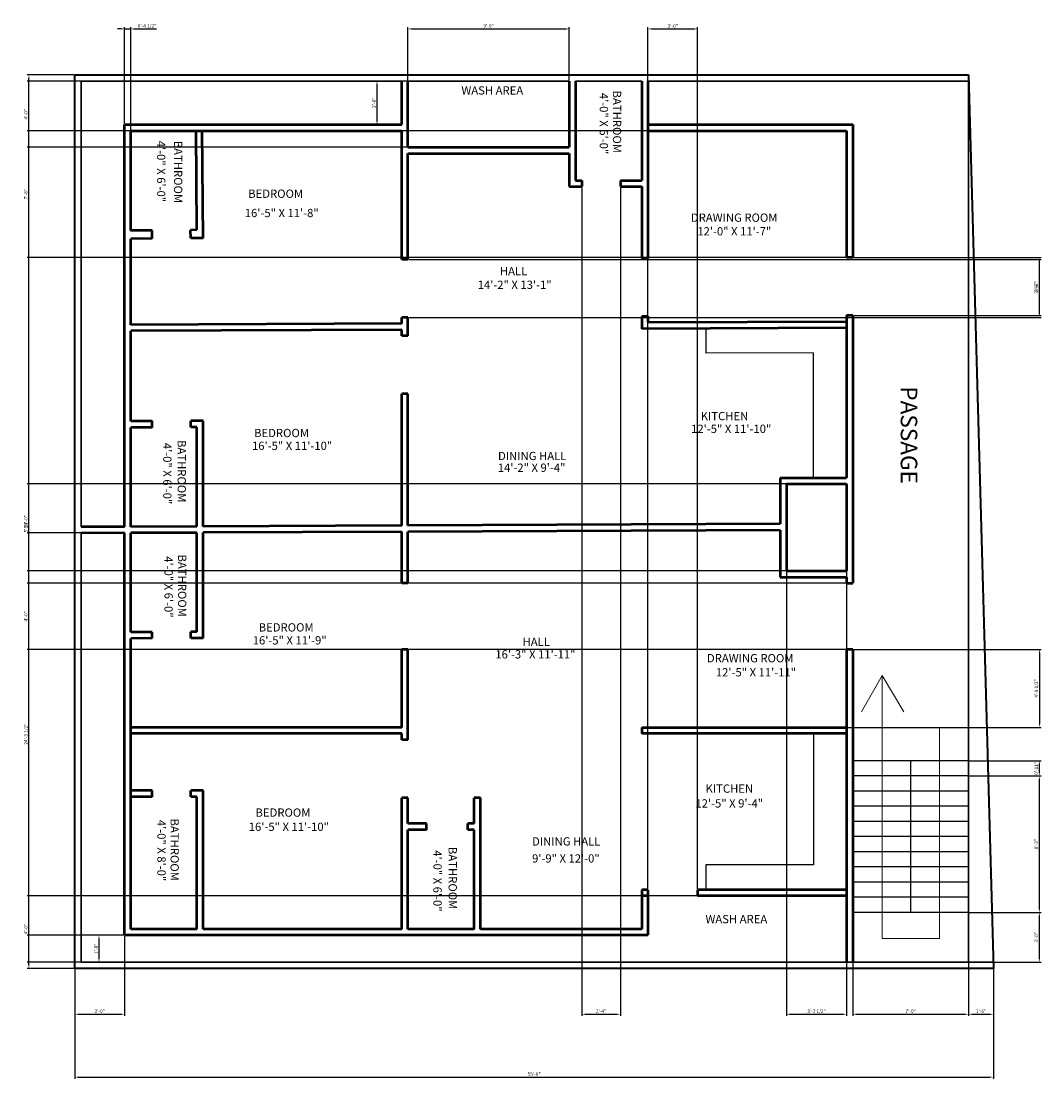
# Model space of a CAD drawing. Units: inches. Extents: x 1269 to 2009, y 1079 to 1846.
import ezdxf

# ---------------------------------------------------------------- set-up
doc = ezdxf.new("R2010")
doc.units = ezdxf.units.IN
for name, color, linetype, lineweight in [('A-ANNO-DIMS', 2, 'Continuous', 18), ('A-ANNO-SYMB', 2, 'Continuous', 18), ('A-ANNO-TEXT', 3, 'Continuous', 18), ('A-AREA-IDEN', 7, 'Continuous', 25), ('A-FLOR-CASE', 9, 'Continuous', 25), ('A-FLOR-STRS', 7, 'Continuous', 25), ('A-WALL', 7, 'Continuous', 50), ('C-PROP', 3, 'Continuous', 35), ('L-SITE-WALL', 8, 'Continuous', 30)]:
    doc.layers.add(name, color=color, linetype=linetype, lineweight=lineweight)
doc.styles.get("Standard").update_dxf_attribs({"font": 'arial.ttf'})
doc.dimstyles.new('ISO-25', dxfattribs={"dimtxt": 2.5, "dimasz": 2.5, "dimexe": 1.25, "dimexo": 0.625, "dimtad": 1, "dimdec": 0, "dimlunit": 4, "dimtxsty": 'Standard', "dimcen": 2.5, "dimadec": 0, "dimazin": 0, "dimtfac": 1, "dimtdec": 0, "dimtmove": 0, "dimatfit": 3, "dimfxl": 1, "dimarcsym": 0})

# ---------------------------------------------------------------- blocks, each defined once
blk = doc.blocks.new('*D1')
at = {"layer": 'A-ANNO-DIMS', "color": 0, "lineweight": -2, "transparency": 16777216}
for p, q in [((1308.03, 1162.83), (1308.03, 1078.8)), ((1974.03, 1162.83), (1974.03, 1078.8)), ((1310.53, 1080.05), (1971.53, 1080.05))]:
    blk.add_line(p, q, dxfattribs=at)
at = {"layer": 'A-ANNO-DIMS', "color": 0, "transparency": 16777216}
for points in [[(1310.53, 1080.47), (1310.53, 1079.64), (1308.03, 1080.05)], [(1971.53, 1080.47), (1971.53, 1079.64), (1974.03, 1080.05)]]:
    blk.add_solid(points, dxfattribs=at)
at = {"layer": 'Defpoints', "color": 0, "transparency": 16777216}
for p in [(1308.03, 1163.45), (1974.03, 1163.45), (1974.03, 1080.05)]:
    blk.add_point(p, dxfattribs=at)
at = {"layer": 'A-ANNO-DIMS', "color": 0, "transparency": 16777216, "insert": (1641.03, 1081.96), "char_height": 2.5, "attachment_point": 5}
blk.add_mtext('55\'-6"', dxfattribs=at)
blk = doc.blocks.new('*D2')
at = {"layer": 'A-ANNO-DIMS', "color": 0, "lineweight": -2, "transparency": 16777216}
for p, q in [((1343.41, 1182.95), (1324.26, 1182.95)), ((1325.51, 1180.45), (1325.51, 1165.95)), ((1343.41, 1163.45), (1324.26, 1163.45))]:
    blk.add_line(p, q, dxfattribs=at)
at = {"layer": 'A-ANNO-DIMS', "color": 0, "transparency": 16777216}
for points in [[(1325.1, 1180.45), (1325.93, 1180.45), (1325.51, 1182.95)], [(1325.1, 1165.95), (1325.93, 1165.95), (1325.51, 1163.45)]]:
    blk.add_solid(points, dxfattribs=at)
at = {"layer": 'Defpoints', "color": 0, "transparency": 16777216}
for p in [(1344.03, 1182.95), (1325.51, 1163.45), (1344.03, 1163.45)]:
    blk.add_point(p, dxfattribs=at)
at = {"layer": 'A-ANNO-DIMS', "color": 0, "transparency": 16777216, "insert": (1323.61, 1173.2), "char_height": 2.5, "attachment_point": 5, "rotation": 90}
blk.add_mtext('1\'-8"', dxfattribs=at)
blk = doc.blocks.new('*D3')
at = {"layer": 'A-ANNO-DIMS', "color": 0, "lineweight": -2, "transparency": 16777216}
for p, q in [((1544.41, 1802.45), (1525.84, 1802.45)), ((1527.09, 1799.95), (1527.09, 1773.45)), ((1544.41, 1770.95), (1525.84, 1770.95))]:
    blk.add_line(p, q, dxfattribs=at)
at = {"layer": 'A-ANNO-DIMS', "color": 0, "transparency": 16777216}
for points in [[(1526.67, 1799.95), (1527.51, 1799.95), (1527.09, 1802.45)], [(1526.67, 1773.45), (1527.51, 1773.45), (1527.09, 1770.95)]]:
    blk.add_solid(points, dxfattribs=at)
at = {"layer": 'Defpoints', "color": 0, "transparency": 16777216}
for p in [(1545.03, 1802.45), (1527.09, 1770.95), (1545.03, 1770.95)]:
    blk.add_point(p, dxfattribs=at)
at = {"layer": 'A-ANNO-DIMS', "color": 0, "transparency": 16777216, "insert": (1525.19, 1786.7), "char_height": 2.5, "attachment_point": 5, "rotation": 90}
blk.add_mtext('2\'-8"', dxfattribs=at)
blk = doc.blocks.new('*D4')
at = {"layer": 'A-ANNO-DIMS', "color": 0, "lineweight": -2, "transparency": 16777216}
for p, q in [((1307.41, 1806.95), (1273.48, 1806.95)), ((1274.73, 1161.45), (1274.73, 1804.45)), ((1307.41, 1158.95), (1273.48, 1158.95))]:
    blk.add_line(p, q, dxfattribs=at)
at = {"layer": 'A-ANNO-DIMS', "color": 0, "transparency": 16777216}
for points in [[(1274.31, 1804.45), (1275.14, 1804.45), (1274.73, 1806.95)], [(1274.31, 1161.45), (1275.14, 1161.45), (1274.73, 1158.95)]]:
    blk.add_solid(points, dxfattribs=at)
at = {"layer": 'Defpoints', "color": 0, "transparency": 16777216}
for p in [(1274.73, 1806.95), (1308.03, 1806.95), (1308.03, 1158.95)]:
    blk.add_point(p, dxfattribs=at)
at = {"layer": 'A-ANNO-DIMS', "color": 0, "transparency": 16777216, "insert": (1272.83, 1482.95), "char_height": 2.5, "attachment_point": 5, "rotation": 90}
blk.add_mtext('54\'-0"', dxfattribs=at)
blk = doc.blocks.new('*D5')
at = {"layer": 'A-ANNO-DIMS', "color": 0, "lineweight": -2, "transparency": 16777216}
for p, q in [((1344.03, 1182.33), (1344.03, 1124.4)), ((1308.03, 1158.33), (1308.03, 1124.4)), ((1310.53, 1125.65), (1341.53, 1125.65))]:
    blk.add_line(p, q, dxfattribs=at)
at = {"layer": 'A-ANNO-DIMS', "color": 0, "transparency": 16777216}
for points in [[(1310.53, 1126.06), (1310.53, 1125.23), (1308.03, 1125.65)], [(1341.53, 1126.06), (1341.53, 1125.23), (1344.03, 1125.65)]]:
    blk.add_solid(points, dxfattribs=at)
at = {"layer": 'Defpoints', "color": 0, "transparency": 16777216}
for p in [(1344.03, 1182.95), (1308.03, 1158.95), (1344.03, 1125.65)]:
    blk.add_point(p, dxfattribs=at)
at = {"layer": 'A-ANNO-DIMS', "color": 0, "transparency": 16777216, "insert": (1326.03, 1127.55), "char_height": 2.5, "attachment_point": 5}
blk.add_mtext('3\'-0"', dxfattribs=at)
blk = doc.blocks.new('*D6')
at = {"layer": 'A-ANNO-DIMS', "color": 0, "lineweight": -2, "transparency": 16777216}
for p, q in [((1872.03, 1162.83), (1872.03, 1124.4)), ((1956.03, 1162.83), (1956.03, 1124.4)), ((1874.53, 1125.65), (1953.53, 1125.65))]:
    blk.add_line(p, q, dxfattribs=at)
at = {"layer": 'A-ANNO-DIMS', "color": 0, "transparency": 16777216}
for points in [[(1874.53, 1126.06), (1874.53, 1125.23), (1872.03, 1125.65)], [(1953.53, 1126.06), (1953.53, 1125.23), (1956.03, 1125.65)]]:
    blk.add_solid(points, dxfattribs=at)
at = {"layer": 'Defpoints', "color": 0, "transparency": 16777216}
for p in [(1872.03, 1163.45), (1956.03, 1163.45), (1956.03, 1125.65)]:
    blk.add_point(p, dxfattribs=at)
at = {"layer": 'A-ANNO-DIMS', "color": 0, "transparency": 16777216, "insert": (1914.03, 1127.55), "char_height": 2.5, "attachment_point": 5}
blk.add_mtext('7\'-0"', dxfattribs=at)
blk = doc.blocks.new('*D7')
at = {"layer": 'A-ANNO-DIMS', "color": 0, "lineweight": -2, "transparency": 16777216}
for p, q in [((1956.03, 1162.83), (1956.03, 1124.4)), ((1974.03, 1162.83), (1974.03, 1124.4)), ((1958.53, 1125.65), (1971.53, 1125.65))]:
    blk.add_line(p, q, dxfattribs=at)
at = {"layer": 'A-ANNO-DIMS', "color": 0, "transparency": 16777216}
for points in [[(1958.53, 1126.06), (1958.53, 1125.23), (1956.03, 1125.65)], [(1971.53, 1126.06), (1971.53, 1125.23), (1974.03, 1125.65)]]:
    blk.add_solid(points, dxfattribs=at)
at = {"layer": 'Defpoints', "color": 0, "transparency": 16777216}
for p in [(1956.03, 1163.45), (1974.03, 1163.45), (1974.03, 1125.65)]:
    blk.add_point(p, dxfattribs=at)
at = {"layer": 'A-ANNO-DIMS', "color": 0, "transparency": 16777216, "insert": (1965.03, 1127.55), "char_height": 2.5, "attachment_point": 5}
blk.add_mtext('1\'-6"', dxfattribs=at)
blk = doc.blocks.new('*D8')
at = {"layer": 'A-ANNO-DIMS', "color": 0, "lineweight": -2, "transparency": 16777216}
for p, q in [((1343.41, 1474.7), (1273.48, 1474.7)), ((1274.73, 1185.45), (1274.73, 1472.2)), ((1343.41, 1182.95), (1273.48, 1182.95))]:
    blk.add_line(p, q, dxfattribs=at)
at = {"layer": 'A-ANNO-DIMS', "color": 0, "transparency": 16777216}
for points in [[(1274.31, 1472.2), (1275.14, 1472.2), (1274.73, 1474.7)], [(1274.31, 1185.45), (1275.14, 1185.45), (1274.73, 1182.95)]]:
    blk.add_solid(points, dxfattribs=at)
at = {"layer": 'Defpoints', "color": 0, "transparency": 16777216}
for p in [(1274.73, 1474.7), (1344.03, 1474.7), (1344.03, 1182.95)]:
    blk.add_point(p, dxfattribs=at)
at = {"layer": 'A-ANNO-DIMS', "color": 0, "transparency": 16777216, "insert": (1272.81, 1328.83), "char_height": 2.5, "attachment_point": 5, "rotation": 90}
blk.add_mtext('24\'-3 1/2"', dxfattribs=at)
blk = doc.blocks.new('*D9')
at = {"layer": 'A-ANNO-DIMS', "color": 0, "lineweight": -2, "transparency": 16777216}
for p, q in [((1956.66, 1298.45), (2008.58, 1298.45)), ((2007.33, 1201.95), (2007.33, 1295.95)), ((1956.66, 1199.45), (2008.58, 1199.45))]:
    blk.add_line(p, q, dxfattribs=at)
at = {"layer": 'A-ANNO-DIMS', "color": 0, "transparency": 16777216}
for points in [[(2006.92, 1295.95), (2007.75, 1295.95), (2007.33, 1298.45)], [(2006.92, 1201.95), (2007.75, 1201.95), (2007.33, 1199.45)]]:
    blk.add_solid(points, dxfattribs=at)
at = {"layer": 'Defpoints', "color": 0, "transparency": 16777216}
for p in [(1956.03, 1298.45), (2007.33, 1298.45), (1956.03, 1199.45)]:
    blk.add_point(p, dxfattribs=at)
at = {"layer": 'A-ANNO-DIMS', "color": 0, "transparency": 16777216, "insert": (2005.43, 1248.95), "char_height": 2.5, "attachment_point": 5, "rotation": 90}
blk.add_mtext('8\'-3"', dxfattribs=at)
blk = doc.blocks.new('*D10')
at = {"layer": 'A-ANNO-DIMS', "color": 0, "lineweight": -2, "transparency": 16777216}
for p, q in [((1956.66, 1199.45), (2008.58, 1199.45)), ((2007.33, 1165.95), (2007.33, 1196.95)), ((1956.66, 1163.45), (2008.58, 1163.45))]:
    blk.add_line(p, q, dxfattribs=at)
at = {"layer": 'A-ANNO-DIMS', "color": 0, "transparency": 16777216}
for points in [[(2006.92, 1196.95), (2007.75, 1196.95), (2007.33, 1199.45)], [(2006.92, 1165.95), (2007.75, 1165.95), (2007.33, 1163.45)]]:
    blk.add_solid(points, dxfattribs=at)
at = {"layer": 'Defpoints', "color": 0, "transparency": 16777216}
for p in [(1956.03, 1199.45), (2007.33, 1199.45), (1956.03, 1163.45)]:
    blk.add_point(p, dxfattribs=at)
at = {"layer": 'A-ANNO-DIMS', "color": 0, "transparency": 16777216, "insert": (2005.43, 1181.45), "char_height": 2.5, "attachment_point": 5, "rotation": 90}
blk.add_mtext('3\'-0"', dxfattribs=at)
blk = doc.blocks.new('*D11')
at = {"layer": 'A-ANNO-DIMS', "color": 0, "lineweight": -2, "transparency": 16777216}
for p, q in [((1872.66, 1674.45), (2008.58, 1674.45)), ((2007.33, 1634.95), (2007.33, 1671.95)), ((1872.66, 1632.45), (2008.58, 1632.45))]:
    blk.add_line(p, q, dxfattribs=at)
at = {"layer": 'A-ANNO-DIMS', "color": 0, "transparency": 16777216}
for points in [[(2006.92, 1671.95), (2007.75, 1671.95), (2007.33, 1674.45)], [(2006.92, 1634.95), (2007.75, 1634.95), (2007.33, 1632.45)]]:
    blk.add_solid(points, dxfattribs=at)
at = {"layer": 'Defpoints', "color": 0, "transparency": 16777216}
for p in [(1872.03, 1674.45), (2007.33, 1674.45), (1872.03, 1632.45)]:
    blk.add_point(p, dxfattribs=at)
at = {"layer": 'A-ANNO-DIMS', "color": 0, "transparency": 16777216, "insert": (2005.43, 1653.45), "char_height": 2.5, "attachment_point": 5, "rotation": 90}
blk.add_mtext('3\'-6"', dxfattribs=at)
blk = doc.blocks.new('*D12')
at = {"layer": 'A-ANNO-DIMS', "color": 0, "lineweight": -2, "transparency": 16777216}
for p, q in [((1866.91, 1766.45), (1273.48, 1766.45)), ((1274.73, 1676.93), (1274.73, 1763.95)), ((1866.91, 1674.43), (1273.48, 1674.43))]:
    blk.add_line(p, q, dxfattribs=at)
at = {"layer": 'A-ANNO-DIMS', "color": 0, "transparency": 16777216}
for points in [[(1274.31, 1763.95), (1275.14, 1763.95), (1274.73, 1766.45)], [(1274.31, 1676.93), (1275.14, 1676.93), (1274.73, 1674.43)]]:
    blk.add_solid(points, dxfattribs=at)
at = {"layer": 'Defpoints', "color": 0, "transparency": 16777216}
for p in [(1274.73, 1766.45), (1867.53, 1766.45), (1867.53, 1674.43)]:
    blk.add_point(p, dxfattribs=at)
at = {"layer": 'A-ANNO-DIMS', "color": 0, "transparency": 16777216, "insert": (1272.83, 1720.44), "char_height": 2.5, "attachment_point": 5, "rotation": 90}
blk.add_mtext('7\'-8"', dxfattribs=at)
blk = doc.blocks.new('*D13')
at = {"layer": 'A-ANNO-DIMS', "color": 0, "lineweight": -2, "transparency": 16777216}
for p, q in [((1866.91, 1438.27), (1273.48, 1438.27)), ((1274.73, 1392.77), (1274.73, 1435.77)), ((1866.91, 1390.27), (1273.48, 1390.27))]:
    blk.add_line(p, q, dxfattribs=at)
at = {"layer": 'A-ANNO-DIMS', "color": 0, "transparency": 16777216}
for points in [[(1274.31, 1435.77), (1275.14, 1435.77), (1274.73, 1438.27)], [(1274.31, 1392.77), (1275.14, 1392.77), (1274.73, 1390.27)]]:
    blk.add_solid(points, dxfattribs=at)
at = {"layer": 'Defpoints', "color": 0, "transparency": 16777216}
for p in [(1274.73, 1438.27), (1867.53, 1438.27), (1867.53, 1390.27)]:
    blk.add_point(p, dxfattribs=at)
at = {"layer": 'A-ANNO-DIMS', "color": 0, "transparency": 16777216, "insert": (1272.83, 1414.27), "char_height": 2.5, "attachment_point": 5, "rotation": 90}
blk.add_mtext('4\'-0"', dxfattribs=at)
blk = doc.blocks.new('*D14')
at = {"layer": 'A-ANNO-DIMS', "color": 0, "lineweight": -2, "transparency": 16777216}
for p, q in [((1868.16, 1390.27), (2008.58, 1390.27)), ((2007.33, 1387.77), (2007.33, 1336.2)), ((1868.16, 1333.7), (2008.58, 1333.7))]:
    blk.add_line(p, q, dxfattribs=at)
at = {"layer": 'A-ANNO-DIMS', "color": 0, "transparency": 16777216}
for points in [[(2006.92, 1387.77), (2007.75, 1387.77), (2007.33, 1390.27)], [(2006.92, 1336.2), (2007.75, 1336.2), (2007.33, 1333.7)]]:
    blk.add_solid(points, dxfattribs=at)
at = {"layer": 'Defpoints', "color": 0, "transparency": 16777216}
for p in [(1867.53, 1390.27), (1867.53, 1333.7), (2007.33, 1333.7)]:
    blk.add_point(p, dxfattribs=at)
at = {"layer": 'A-ANNO-DIMS', "color": 0, "transparency": 16777216, "insert": (2005.42, 1361.99), "char_height": 2.5, "attachment_point": 5, "rotation": 90}
blk.add_mtext('4\'-8 1/2"', dxfattribs=at)
blk = doc.blocks.new('*D15')
at = {"layer": 'A-ANNO-DIMS', "color": 0, "lineweight": -2, "transparency": 16777216}
for p, q in [((1675.53, 1725.33), (1675.53, 1124.4)), ((1703.53, 1725.33), (1703.53, 1124.4)), ((1678.03, 1125.65), (1701.03, 1125.65))]:
    blk.add_line(p, q, dxfattribs=at)
at = {"layer": 'A-ANNO-DIMS', "color": 0, "transparency": 16777216}
for points in [[(1678.03, 1126.06), (1678.03, 1125.23), (1675.53, 1125.65)], [(1701.03, 1126.06), (1701.03, 1125.23), (1703.53, 1125.65)]]:
    blk.add_solid(points, dxfattribs=at)
at = {"layer": 'Defpoints', "color": 0, "transparency": 16777216}
for p in [(1675.53, 1725.95), (1703.53, 1725.95), (1703.53, 1125.65)]:
    blk.add_point(p, dxfattribs=at)
at = {"layer": 'A-ANNO-DIMS', "color": 0, "transparency": 16777216, "insert": (1689.53, 1127.53), "char_height": 2.5, "attachment_point": 5}
blk.add_mtext('2\'-4"', dxfattribs=at)
blk = doc.blocks.new('*D16')
at = {"layer": 'A-ANNO-DIMS', "color": 0, "lineweight": -2, "transparency": 16777216}
for p, q in [((1549.53, 1803.08), (1549.53, 1841.5)), ((1666.53, 1803.08), (1666.53, 1841.5)), ((1552.03, 1840.25), (1664.03, 1840.25))]:
    blk.add_line(p, q, dxfattribs=at)
at = {"layer": 'A-ANNO-DIMS', "color": 0, "transparency": 16777216}
for points in [[(1552.03, 1840.67), (1552.03, 1839.84), (1549.53, 1840.25)], [(1664.03, 1840.67), (1664.03, 1839.84), (1666.53, 1840.25)]]:
    blk.add_solid(points, dxfattribs=at)
at = {"layer": 'Defpoints', "color": 0, "transparency": 16777216}
for p in [(1666.53, 1840.25), (1549.53, 1802.45), (1666.53, 1802.45)]:
    blk.add_point(p, dxfattribs=at)
at = {"layer": 'A-ANNO-DIMS', "color": 0, "transparency": 16777216, "insert": (1608.03, 1842.16), "char_height": 2.5, "attachment_point": 5}
blk.add_mtext('9\'-9"', dxfattribs=at)
blk = doc.blocks.new('*D17')
at = {"layer": 'A-ANNO-DIMS', "color": 0, "lineweight": -2, "transparency": 16777216}
for p, q in [((1665.91, 1802.45), (1273.48, 1802.45)), ((1274.73, 1756.95), (1274.73, 1799.95)), ((1665.91, 1754.45), (1273.48, 1754.45))]:
    blk.add_line(p, q, dxfattribs=at)
at = {"layer": 'A-ANNO-DIMS', "color": 0, "transparency": 16777216}
for points in [[(1274.31, 1799.95), (1275.14, 1799.95), (1274.73, 1802.45)], [(1274.31, 1756.95), (1275.14, 1756.95), (1274.73, 1754.45)]]:
    blk.add_solid(points, dxfattribs=at)
at = {"layer": 'Defpoints', "color": 0, "transparency": 16777216}
for p in [(1274.73, 1802.45), (1666.53, 1802.45), (1666.53, 1754.45)]:
    blk.add_point(p, dxfattribs=at)
at = {"layer": 'A-ANNO-DIMS', "color": 0, "transparency": 16777216, "insert": (1272.83, 1778.45), "char_height": 2.5, "attachment_point": 5, "rotation": 90}
blk.add_mtext('4\'-0"', dxfattribs=at)
blk = doc.blocks.new('*D18')
at = {"layer": 'A-ANNO-DIMS', "color": 0, "lineweight": -2, "transparency": 16777216}
for p, q in [((1723.53, 1216.58), (1723.53, 1841.5)), ((1759.53, 1216.58), (1759.53, 1841.5)), ((1726.03, 1840.25), (1757.03, 1840.25))]:
    blk.add_line(p, q, dxfattribs=at)
at = {"layer": 'A-ANNO-DIMS', "color": 0, "transparency": 16777216}
for points in [[(1726.03, 1840.67), (1726.03, 1839.84), (1723.53, 1840.25)], [(1757.03, 1840.67), (1757.03, 1839.84), (1759.53, 1840.25)]]:
    blk.add_solid(points, dxfattribs=at)
at = {"layer": 'Defpoints', "color": 0, "transparency": 16777216}
for p in [(1759.53, 1840.25), (1723.53, 1215.95), (1759.53, 1215.95)]:
    blk.add_point(p, dxfattribs=at)
at = {"layer": 'A-ANNO-DIMS', "color": 0, "transparency": 16777216, "insert": (1741.53, 1842.16), "char_height": 2.5, "attachment_point": 5}
blk.add_mtext('3\'-0"', dxfattribs=at)
blk = doc.blocks.new('*D19')
at = {"layer": 'A-ANNO-DIMS', "color": 0, "lineweight": -2, "transparency": 16777216}
for p, q in [((1956.66, 1309.45), (2008.58, 1309.45)), ((2007.33, 1300.95), (2007.33, 1306.95)), ((1956.66, 1298.45), (2008.58, 1298.45))]:
    blk.add_line(p, q, dxfattribs=at)
at = {"layer": 'A-ANNO-DIMS', "color": 0, "transparency": 16777216}
for points in [[(2006.92, 1306.95), (2007.75, 1306.95), (2007.33, 1309.45)], [(2006.92, 1300.95), (2007.75, 1300.95), (2007.33, 1298.45)]]:
    blk.add_solid(points, dxfattribs=at)
at = {"layer": 'Defpoints', "color": 0, "transparency": 16777216}
for p in [(1956.03, 1309.45), (2007.33, 1309.45), (1956.03, 1298.45)]:
    blk.add_point(p, dxfattribs=at)
at = {"layer": 'A-ANNO-DIMS', "color": 0, "transparency": 16777216, "insert": (2005.43, 1303.95), "char_height": 2.5, "attachment_point": 5, "rotation": 90}
blk.add_mtext('0\'-11"', dxfattribs=at)
blk = doc.blocks.new('*D20')
at = {"layer": 'A-ANNO-DIMS', "color": 0, "lineweight": -2, "transparency": 16777216}
for p, q in [((1344.03, 1771.58), (1344.03, 1841.5)), ((1348.53, 1767.08), (1348.53, 1841.5)), ((1341.53, 1840.25), (1339.03, 1840.25)), ((1344.03, 1840.25), (1348.53, 1840.25)), ((1351.03, 1840.25), (1367.25, 1840.25))]:
    blk.add_line(p, q, dxfattribs=at)
at = {"layer": 'A-ANNO-DIMS', "color": 0, "transparency": 16777216}
for points in [[(1341.53, 1840.67), (1341.53, 1839.84), (1344.03, 1840.25)], [(1351.03, 1840.67), (1351.03, 1839.84), (1348.53, 1840.25)]]:
    blk.add_solid(points, dxfattribs=at)
at = {"layer": 'Defpoints', "color": 0, "transparency": 16777216}
for p in [(1348.53, 1840.25), (1344.03, 1770.95), (1348.53, 1766.45)]:
    blk.add_point(p, dxfattribs=at)
at = {"layer": 'A-ANNO-DIMS', "color": 0, "transparency": 16777216, "insert": (1360.39, 1842.17), "char_height": 2.5, "attachment_point": 5}
blk.add_mtext('0\'-4 1/2"', dxfattribs=at)
blk = doc.blocks.new('*D21')
at = {"layer": 'A-ANNO-DIMS', "color": 0, "lineweight": -2, "transparency": 16777216}
for p, q in [((1824.03, 1509.65), (1824.03, 1124.4)), ((1867.53, 1509.65), (1867.53, 1124.4)), ((1826.53, 1125.65), (1865.03, 1125.65))]:
    blk.add_line(p, q, dxfattribs=at)
at = {"layer": 'A-ANNO-DIMS', "color": 0, "transparency": 16777216}
for points in [[(1826.53, 1126.06), (1826.53, 1125.23), (1824.03, 1125.65)], [(1865.03, 1126.06), (1865.03, 1125.23), (1867.53, 1125.65)]]:
    blk.add_solid(points, dxfattribs=at)
at = {"layer": 'Defpoints', "color": 0, "transparency": 16777216}
for p in [(1824.03, 1510.27), (1867.53, 1510.27), (1867.53, 1125.65)]:
    blk.add_point(p, dxfattribs=at)
at = {"layer": 'A-ANNO-DIMS', "color": 0, "transparency": 16777216, "insert": (1845.78, 1127.57), "char_height": 2.5, "attachment_point": 5}
blk.add_mtext('3\'-7 1/2"', dxfattribs=at)
blk = doc.blocks.new('*D22')
at = {"layer": 'A-ANNO-DIMS', "color": 0, "lineweight": -2, "transparency": 16777216}
for p, q in [((1866.91, 1510.27), (1273.48, 1510.27)), ((1274.73, 1449.77), (1274.73, 1507.77)), ((1866.91, 1447.27), (1273.48, 1447.27))]:
    blk.add_line(p, q, dxfattribs=at)
at = {"layer": 'A-ANNO-DIMS', "color": 0, "transparency": 16777216}
for points in [[(1274.31, 1507.77), (1275.14, 1507.77), (1274.73, 1510.27)], [(1274.31, 1449.77), (1275.14, 1449.77), (1274.73, 1447.27)]]:
    blk.add_solid(points, dxfattribs=at)
at = {"layer": 'Defpoints', "color": 0, "transparency": 16777216}
for p in [(1274.73, 1510.27), (1867.53, 1510.27), (1867.53, 1447.27)]:
    blk.add_point(p, dxfattribs=at)
at = {"layer": 'A-ANNO-DIMS', "color": 0, "transparency": 16777216, "insert": (1272.83, 1478.77), "char_height": 2.5, "attachment_point": 5, "rotation": 90}
blk.add_mtext('5\'-3"', dxfattribs=at)
blk = doc.blocks.new('*D23')
at = {"layer": 'A-ANNO-DIMS', "color": 0, "lineweight": -2, "transparency": 16777216}
for p, q in [((1866.91, 1211.45), (1273.48, 1211.45)), ((1274.73, 1165.95), (1274.73, 1208.95)), ((1866.91, 1163.45), (1273.48, 1163.45))]:
    blk.add_line(p, q, dxfattribs=at)
at = {"layer": 'A-ANNO-DIMS', "color": 0, "transparency": 16777216}
for points in [[(1274.31, 1208.95), (1275.14, 1208.95), (1274.73, 1211.45)], [(1274.31, 1165.95), (1275.14, 1165.95), (1274.73, 1163.45)]]:
    blk.add_solid(points, dxfattribs=at)
at = {"layer": 'Defpoints', "color": 0, "transparency": 16777216}
for p in [(1274.73, 1211.45), (1867.53, 1211.45), (1867.53, 1163.45)]:
    blk.add_point(p, dxfattribs=at)
at = {"layer": 'A-ANNO-DIMS', "color": 0, "transparency": 16777216, "insert": (1272.83, 1187.45), "char_height": 2.5, "attachment_point": 5, "rotation": 90}
blk.add_mtext('4\'-0"', dxfattribs=at)
blk = doc.blocks.new('*D24')
at = {"layer": 'A-ANNO-DIMS', "color": 0, "lineweight": -2, "transparency": 16777216}
for p, q in [((1550.16, 1673.08), (2008.58, 1673.08)), ((2007.33, 1633.58), (2007.33, 1670.58)), ((1550.16, 1631.08), (2008.58, 1631.08))]:
    blk.add_line(p, q, dxfattribs=at)
at = {"layer": 'A-ANNO-DIMS', "color": 0, "transparency": 16777216}
for points in [[(2006.92, 1670.58), (2007.75, 1670.58), (2007.33, 1673.08)], [(2006.92, 1633.58), (2007.75, 1633.58), (2007.33, 1631.08)]]:
    blk.add_solid(points, dxfattribs=at)
at = {"layer": 'Defpoints', "color": 0, "transparency": 16777216}
for p in [(1549.53, 1673.08), (2007.33, 1673.08), (1549.53, 1631.08)]:
    blk.add_point(p, dxfattribs=at)
at = {"layer": 'A-ANNO-DIMS', "color": 0, "transparency": 16777216, "insert": (2005.43, 1652.08), "char_height": 2.5, "attachment_point": 5, "rotation": 90}
blk.add_mtext('3\'-6"', dxfattribs=at)

msp = doc.modelspace()

# ---------------------------------------------------------------- linework, layer by layer
at = {"layer": 'A-ANNO-SYMB'}
for p, q in [((1893.29, 1371.22), (1878.37, 1344.95)), ((1893.29, 1180.65), (1893.29, 1371.22)), ((1893.29, 1371.22), (1909.09, 1345.09)), ((1934.88, 1333.66), (1934.88, 1180.65)), ((1934.88, 1180.65), (1893.29, 1180.65))]:
    msp.add_line(p, q, dxfattribs=at)
at = {"layer": 'A-FLOR-CASE'}
for p, q in [((1765.4, 1623), (1765.4, 1605)), ((1843.4, 1605.33), (1765.4, 1605)), ((1843.4, 1605.33), (1843.4, 1514.77)), ((1843.53, 1329.2), (1843.53, 1233.95)), ((1843.53, 1233.95), (1765.53, 1233.95)), ((1765.53, 1233.95), (1765.53, 1215.95))]:
    msp.add_line(p, q, dxfattribs=at)
at = {"layer": 'A-FLOR-STRS'}
for p, q in [((1956.03, 1309.45), (1872.03, 1309.45)), ((1914.03, 1309.45), (1914.03, 1199.45)), ((1956.03, 1298.45), (1872.03, 1298.45)), ((1956.03, 1287.45), (1872.03, 1287.45)), ((1956.03, 1276.45), (1872.03, 1276.45)), ((1956.03, 1265.45), (1872.03, 1265.45)), ((1956.03, 1254.45), (1872.03, 1254.45)), ((1956.03, 1243.45), (1872.03, 1243.45)), ((1956.03, 1232.45), (1872.03, 1232.45)), ((1956.03, 1221.45), (1872.03, 1221.45)), ((1956.03, 1210.45), (1872.03, 1210.45)), ((1956.03, 1199.45), (1872.03, 1199.45))]:
    msp.add_line(p, q, dxfattribs=at)
at = {"layer": 'A-WALL'}
for p, q in [((1545.03, 1770.95), (1545.03, 1802.45)), ((1549.53, 1754.45), (1549.53, 1802.45)), ((1666.53, 1802.45), (1666.53, 1754.45)), ((1671.03, 1802.45), (1671.03, 1730.45)), ((1719.03, 1802.45), (1719.03, 1730.45)), ((1723.53, 1802.45), (1723.53, 1673.82)), ((1344.03, 1479.2), (1344.03, 1770.95)), ((1344.03, 1770.95), (1545.03, 1770.95)), ((1348.53, 1694.04), (1348.53, 1766.45)), ((1348.53, 1766.45), (1545.03, 1766.45)), ((1396.48, 1694.45), (1395.86, 1766.45)), ((1401.03, 1688.49), (1400.36, 1766.49)), ((1545.03, 1673.06), (1545.03, 1766.45)), ((1723.53, 1770.95), (1872.03, 1770.95)), ((1723.53, 1766.45), (1867.53, 1766.45)), ((1867.53, 1766.45), (1867.53, 1674.43)), ((1872.03, 1770.95), (1872.03, 1674.45)), ((1549.53, 1754.45), (1666.53, 1754.45)), ((1549.53, 1673.08), (1549.53, 1749.95)), ((1549.53, 1749.95), (1666.53, 1749.95)), ((1666.53, 1749.95), (1666.53, 1725.95)), ((1671.03, 1730.45), (1675.53, 1730.45)), ((1675.53, 1730.45), (1675.53, 1725.95)), ((1703.53, 1730.45), (1719.03, 1730.45)), ((1703.53, 1730.45), (1703.53, 1725.95)), ((1666.53, 1725.95), (1675.53, 1725.95)), ((1703.53, 1725.95), (1719.03, 1725.95)), ((1719.03, 1725.95), (1719.03, 1673.8)), ((1363.98, 1694.18), (1348.48, 1694.04)), ((1364.03, 1688.18), (1348.53, 1688.04)), ((1348.53, 1625.72), (1348.53, 1688.04)), ((1364.03, 1688.18), (1363.98, 1694.18)), ((1396.48, 1694.45), (1391.98, 1694.41)), ((1392.03, 1688.42), (1391.98, 1694.41)), ((1401.03, 1688.49), (1392.03, 1688.42)), ((1549.53, 1673.08), (1545.03, 1673.06)), ((1723.53, 1673.82), (1719.03, 1673.8)), ((1872.03, 1674.45), (1867.53, 1674.43)), ((1545.03, 1626.56), (1348.53, 1625.72)), ((1549.53, 1631.08), (1545.03, 1631.06)), ((1545.03, 1626.56), (1545.03, 1631.06)), ((1549.53, 1617.58), (1549.53, 1631.08)), ((1723.53, 1631.82), (1719.03, 1631.8)), ((1719.03, 1631.8), (1719.03, 1622.8)), ((1723.53, 1631.82), (1723.53, 1627.32)), ((1867.53, 1627.93), (1723.53, 1627.32)), ((1872.03, 1632.45), (1867.53, 1632.43)), ((1867.53, 1632.43), (1867.53, 1514.77)), ((1872.03, 1632.45), (1872.03, 1438.27)), ((1545.03, 1622.06), (1348.53, 1621.22)), ((1348.53, 1555.72), (1348.53, 1621.22)), ((1545.03, 1617.56), (1545.03, 1622.06)), ((1867.53, 1623.43), (1719.03, 1622.8)), ((1549.53, 1617.58), (1545.03, 1617.56)), ((1549.53, 1575.58), (1545.03, 1575.56)), ((1545.03, 1480.06), (1545.03, 1575.56)), ((1549.53, 1480.08), (1549.53, 1575.58)), ((1364.03, 1555.79), (1348.53, 1555.72)), ((1364.03, 1551.29), (1348.53, 1551.22)), ((1348.53, 1479.22), (1348.53, 1551.22)), ((1364.03, 1551.29), (1364.03, 1555.93)), ((1401.13, 1555.94), (1392.03, 1555.91)), ((1392.03, 1551.41), (1392.03, 1555.93)), ((1396.53, 1551.43), (1392.03, 1551.41)), ((1396.53, 1479.42), (1396.53, 1551.43)), ((1401.03, 1479.44), (1401.03, 1555.94)), ((1401.13, 1551.44), (1401.03, 1551.44)), ((1819.53, 1514.77), (1819.53, 1481.23)), ((1819.53, 1514.77), (1867.53, 1514.77)), ((1824.03, 1510.27), (1824.03, 1447.27)), ((1824.03, 1510.27), (1867.53, 1510.27)), ((1867.53, 1510.27), (1867.53, 1447.27)), ((1819.53, 1481.23), (1549.53, 1480.08)), ((1344.03, 1479.2), (1312.53, 1479.07)), ((1344.03, 1474.7), (1312.53, 1474.57)), ((1344.03, 1479.2), (1344.02, 1479.2)), ((1344.03, 1182.95), (1344.03, 1474.7)), ((1396.53, 1479.42), (1348.53, 1479.22)), ((1396.53, 1474.92), (1348.53, 1474.72)), ((1348.53, 1402.72), (1348.53, 1474.72)), ((1396.53, 1402.92), (1396.53, 1474.92)), ((1545.03, 1480.06), (1401.03, 1479.44)), ((1545.03, 1475.56), (1401.03, 1474.94)), ((1401.03, 1398.44), (1401.03, 1474.94)), ((1545.03, 1438.27), (1545.03, 1475.56)), ((1819.53, 1476.73), (1549.53, 1475.58)), ((1549.53, 1438.27), (1549.53, 1475.58)), ((1819.53, 1476.73), (1819.53, 1442.77)), ((1872.04, 1476.95), (1872.03, 1476.95)), ((1867.63, 1452.93), (1867.53, 1452.93)), ((1819.53, 1442.77), (1867.53, 1442.77)), ((1824.03, 1447.27), (1867.53, 1447.27)), ((1867.53, 1442.77), (1867.53, 1438.27)), ((1549.53, 1438.27), (1545.03, 1438.27)), ((1867.53, 1438.27), (1872.03, 1438.27)), ((1364.03, 1402.79), (1348.53, 1402.72)), ((1364.03, 1398.29), (1348.53, 1398.22)), ((1348.53, 1187.45), (1348.53, 1398.22)), ((1364.03, 1398.29), (1364.03, 1402.79)), ((1396.53, 1402.92), (1392.03, 1402.9)), ((1392.03, 1398.4), (1392.03, 1402.9)), ((1401.03, 1398.44), (1392.03, 1398.4)), ((1545.03, 1333.7), (1545.03, 1390.27)), ((1549.53, 1390.27), (1545.03, 1390.27)), ((1549.53, 1324.7), (1549.53, 1390.27)), ((1867.53, 1390.27), (1867.53, 1163.45)), ((1872.03, 1390.27), (1867.53, 1390.27)), ((1872.03, 1390.27), (1872.03, 1163.45)), ((1545.03, 1333.7), (1348.53, 1333.7)), ((1545.03, 1329.2), (1348.53, 1329.2)), ((1545.03, 1324.7), (1545.03, 1329.2)), ((1719.03, 1333.7), (1719.03, 1329.2)), ((1719.03, 1333.7), (1867.53, 1333.7)), ((1867.53, 1329.2), (1719.03, 1329.2)), ((1767.04, 1333.7), (1771.54, 1333.7)), ((1549.53, 1324.7), (1545.03, 1324.7)), ((1364.03, 1287.95), (1348.53, 1287.95)), ((1364.03, 1283.45), (1348.53, 1283.45)), ((1364.03, 1283.45), (1364.03, 1287.95)), ((1401.03, 1287.95), (1392.03, 1287.95)), ((1392.03, 1283.45), (1392.03, 1287.95)), ((1396.53, 1283.45), (1392.03, 1283.45)), ((1396.53, 1187.45), (1396.53, 1283.45)), ((1401.03, 1187.45), (1401.03, 1287.95)), ((1549.53, 1282.7), (1545.03, 1282.7)), ((1545.03, 1187.45), (1545.03, 1282.7)), ((1549.53, 1263.95), (1549.53, 1282.7)), ((1602.03, 1282.7), (1597.53, 1282.7)), ((1597.53, 1263.95), (1597.53, 1282.7)), ((1602.03, 1187.45), (1602.03, 1282.7)), ((1563.03, 1263.95), (1549.53, 1263.95)), ((1563.03, 1259.45), (1549.53, 1259.45)), ((1549.53, 1187.45), (1549.53, 1259.45)), ((1563.03, 1259.45), (1563.03, 1263.95)), ((1597.53, 1263.95), (1593.03, 1263.95)), ((1593.03, 1259.45), (1593.03, 1263.95)), ((1597.53, 1259.45), (1593.03, 1259.45)), ((1597.53, 1187.45), (1597.53, 1259.45)), ((1723.53, 1215.95), (1719.03, 1215.95)), ((1719.03, 1215.95), (1719.03, 1187.45)), ((1723.53, 1215.95), (1723.53, 1182.95)), ((1867.53, 1215.95), (1759.53, 1215.95)), ((1759.53, 1215.95), (1759.53, 1211.45)), ((1723.53, 1211.45), (1719.03, 1211.45)), ((1867.53, 1211.45), (1759.53, 1211.45)), ((1723.53, 1182.95), (1344.03, 1182.95)), ((1396.53, 1187.45), (1348.53, 1187.45)), ((1545.03, 1187.45), (1401.03, 1187.45)), ((1597.53, 1187.45), (1549.53, 1187.45)), ((1719.03, 1187.45), (1602.03, 1187.45))]:
    msp.add_line(p, q, dxfattribs=at)
at = {"layer": 'C-PROP'}
for p, q in [((1308.03, 1158.95), (1308.03, 1806.95)), ((1308.03, 1806.95), (1956.03, 1806.95)), ((1956.03, 1806.95), (1974.03, 1158.95)), ((1974.03, 1158.95), (1308.03, 1158.95))]:
    msp.add_line(p, q, dxfattribs=at)
at = {"layer": 'L-SITE-WALL'}
for p, q in [((1956.03, 1806.95), (1956.03, 1163.45)), ((1312.53, 1479.07), (1312.53, 1802.45)), ((1312.53, 1802.45), (1545.03, 1802.45)), ((1549.53, 1802.45), (1666.53, 1802.45)), ((1671.03, 1802.45), (1719.03, 1802.45)), ((1723.53, 1802.45), (1956.03, 1802.45)), ((1312.53, 1163.45), (1312.53, 1474.57)), ((1974.03, 1163.45), (1312.53, 1163.45))]:
    msp.add_line(p, q, dxfattribs=at)

# ---------------------------------------------------------------- texts
at = {"layer": 'A-ANNO-TEXT', "char_height": 6, "attachment_point": 1, "rotation": 270}
for s, width, insert in [('4\'-0" X 6\'-0"', 45.2228, (1694.59, 1793.9)), ('4\'-0" X 6\'-0"', 45.2228, (1373.57, 1759.17)), ('4\'-0" X 6\'-0"', 45.2228, (1378.07, 1540.05)), ('4\'-0" X 6\'-0"', 45.2228, (1378.99, 1457.83)), ('4\'-0" X 8\'-0"', 47.7154, (1373.86, 1266.64)), ('4\'-0" X 6\'-0"', 45.2228, (1573.99, 1244.61))]:
    msp.add_mtext_dynamic_manual_height_columns(s, width=width, gutter_width=12.5, heights=[0], dxfattribs=dict(at, insert=insert))
at = {"layer": 'A-ANNO-TEXT', "char_height": 6, "attachment_point": 1}
for s, width, insert in [('16\'-5" X 11\'-8"', 58.2006, (1431.23, 1709.75)), ('12\'-0" X 11\'-7"', 53.9923, (1759.35, 1696.5)), ('14\'-2" X 13\'-1"', 53.9923, (1600.09, 1657.68)), ('12\'-5" X 11\'-10"', 61.4849, (1754.85, 1553.22)), ('16\'-5" X 11\'-10"', 66.6765, (1436.46, 1540.92)), ('14\'-2" X 9\'-4"', 53.9923, (1614.66, 1525.04)), ('16\'-5" X 11\'-9"', 53.9923, (1436.99, 1399.83)), ('16\'-3" X 11\'-11"', 67.0938, (1612.88, 1389.69)), ('12\'-5" X 11\'-11"', 67.0938, (1772.79, 1376.67)), ('12\'-5" X 9\'-4"', 53.9923, (1757.98, 1281.58)), ('16\'-5" X 11\'-10"', 66.5223, (1434.11, 1264.61)), ('9\'-9" X 12\'-0"', 53.9923, (1639.52, 1241.66))]:
    msp.add_mtext_dynamic_manual_height_columns(s, width=width, gutter_width=12.5, heights=[0], dxfattribs=dict(at, insert=insert))
at = {"layer": 'A-AREA-IDEN', "char_height": 6, "attachment_point": 1}
for s, width, insert in [('WASH AREA', 45.6881, (1588.28, 1798.66)), ('BEDROOM', 84.3796, (1433.71, 1723.75)), ('\\pxqc;DRAWING ROOM', 84.3796, (1743.88, 1706.38)), ('HALL', 45.6881, (1616.17, 1667.62)), ('KITCHEN', 45.6881, (1761.79, 1562.46)), ('BEDROOM', 84.3796, (1437.97, 1550.21)), ('DINING HALL', 71.8252, (1614.84, 1533.53)), ('BEDROOM', 84.3796, (1441.31, 1409.23)), ('HALL', 45.6881, (1632.63, 1398.71)), ('\\pxqc;DRAWING ROOM', 84.3796, (1755.51, 1386.9)), ('KITCHEN', 45.6881, (1765.29, 1292.31)), ('BEDROOM', 84.3796, (1439, 1274.92)), ('DINING HALL', 71.23, (1639.52, 1253.99)), ('WASH AREA', 45.6881, (1765.25, 1197.65))]:
    msp.add_mtext_dynamic_manual_height_columns(s, width=width, gutter_width=12.5, heights=[0], dxfattribs=dict(at, insert=insert))
at = {"layer": 'A-AREA-IDEN', "attachment_point": 1, "rotation": 270}
for s, width, insert, char_height in [('BATHROOM', 56.2032, (1704.15, 1795.52), 6), ('BATHROOM', 56.2032, (1385.91, 1759.17), 6), ('\\pxsm1,qc;{\\T4;PASSAGE}', 291.8093, (1918.83, 1691.59), 12), ('BATHROOM', 56.2032, (1388.52, 1542.1), 6), ('BATHROOM', 56.2032, (1388.84, 1459.07), 6), ('BATHROOM', 56.2032, (1383.38, 1267.59), 6), ('BATHROOM', 56.2032, (1584.98, 1246.98), 6)]:
    msp.add_mtext_dynamic_manual_height_columns(s, width=width, gutter_width=12.5, heights=[0], dxfattribs=dict(at, insert=insert, char_height=char_height))

# ---------------------------------------------------------------- dimensions: what is measured, and where the dimension line sits
at = {"layer": 'A-ANNO-DIMS'}
for base, p1, p2, override, picture, middle in [((1348.53, 1840.25), (1344.03, 1770.95), (1348.53, 1766.45), {"dimdec": 1, "dimlfac": 1, "dimrnd": 0, "dimzin": 1, "dimdsep": 46, "dimlunit": 4, "dimfrac": 2}, '*D20', (1360.39, 1842.17)), ((1666.53, 1840.25), (1549.53, 1802.45), (1666.53, 1802.45), {"dimdec": 1, "dimlfac": 1, "dimrnd": 0, "dimzin": 1, "dimdsep": 46, "dimlunit": 4, "dimfrac": 2}, '*D16', (1608.03, 1842.16)), ((1759.53, 1840.25), (1723.53, 1215.95), (1759.53, 1215.95), {"dimdec": 1, "dimlfac": 1, "dimrnd": 0, "dimzin": 1, "dimdsep": 46, "dimlunit": 4, "dimfrac": 2}, '*D18', (1741.53, 1842.16)), ((1703.53, 1125.65), (1675.53, 1725.95), (1703.53, 1725.95), {"dimdec": 1, "dimlfac": 1, "dimrnd": 0, "dimzin": 1, "dimdsep": 46, "dimlunit": 4, "dimfrac": 2}, '*D15', (1689.53, 1127.53)), ((1867.53, 1125.65), (1824.03, 1510.27), (1867.53, 1510.27), {"dimdec": 1, "dimlfac": 1, "dimrnd": 0, "dimzin": 1, "dimdsep": 46, "dimlunit": 4, "dimfrac": 2}, '*D21', (1845.78, 1127.57)), ((1344.03, 1125.65), (1308.03, 1158.95), (1344.03, 1182.95), {"dimdec": 1, "dimlfac": 1, "dimrnd": 0, "dimzin": 1, "dimdsep": 46, "dimlunit": 4, "dimfrac": 2}, '*D5', (1326.03, 1127.55)), ((1974.03, 1080.05), (1308.03, 1163.45), (1974.03, 1163.45), {"dimclrd": 0, "dimclre": 0, "dimclrt": 0}, '*D1', (1641.03, 1081.96)), ((1956.03, 1125.65), (1872.03, 1163.45), (1956.03, 1163.45), {"dimdec": 1, "dimlfac": 1, "dimrnd": 0, "dimzin": 1, "dimdsep": 46, "dimlunit": 4, "dimfrac": 2}, '*D6', (1914.03, 1127.55)), ((1974.03, 1125.65), (1956.03, 1163.45), (1974.03, 1163.45), {"dimdec": 1, "dimlfac": 1, "dimrnd": 0, "dimzin": 1, "dimdsep": 46, "dimlunit": 4, "dimfrac": 2}, '*D7', (1965.03, 1127.55))]:
    dim = msp.add_linear_dim(base=base, p1=p1, p2=p2, dimstyle='ISO-25', override=override, dxfattribs=at)
    dim.commit()
    dim.dimension.update_dxf_attribs({"geometry": picture, "text_midpoint": middle})
for base, p1, p2, override, picture, middle in [((1274.73, 1806.95), (1308.03, 1158.95), (1308.03, 1806.95), {"dimdec": 1, "dimlfac": 1, "dimrnd": 0, "dimzin": 1, "dimdsep": 46, "dimlunit": 4, "dimfrac": 2}, '*D4', (1272.83, 1482.95)), ((1274.73, 1802.45), (1666.53, 1754.45), (1666.53, 1802.45), {"dimdec": 1, "dimlfac": 1, "dimrnd": 0, "dimzin": 1, "dimdsep": 46, "dimlunit": 4, "dimfrac": 2}, '*D17', (1272.83, 1778.45)), ((1527.08887493, 1770.95062781), (1545.03111399, 1802.45062781), (1545.03111399, 1770.95062781), {"dimclrd": 0, "dimclre": 0, "dimclrt": 0}, '*D3', (1525.18744247, 1786.70062781)), ((1274.73, 1766.45), (1867.53, 1674.43), (1867.53, 1766.45), {"dimdec": 1, "dimlfac": 1, "dimrnd": 0, "dimzin": 1, "dimdsep": 46, "dimlunit": 4, "dimfrac": 2}, '*D12', (1272.83, 1720.44)), ((2007.33, 1673.08), (1549.53, 1631.08), (1549.53, 1673.08), {"dimdec": 1, "dimlfac": 1, "dimrnd": 0, "dimzin": 1, "dimdsep": 46, "dimlunit": 4, "dimfrac": 2}, '*D24', (2005.43, 1652.08)), ((2007.33, 1674.45), (1872.03, 1632.45), (1872.03, 1674.45), {"dimdec": 1, "dimlfac": 1, "dimrnd": 0, "dimzin": 1, "dimdsep": 46, "dimlunit": 4, "dimfrac": 2}, '*D11', (2005.43, 1653.45)), ((1274.73, 1510.27), (1867.53, 1447.27), (1867.53, 1510.27), {"dimdec": 1, "dimlfac": 1, "dimrnd": 0, "dimzin": 1, "dimdsep": 46, "dimlunit": 4, "dimfrac": 2}, '*D22', (1272.83, 1478.77)), ((1274.72811, 1474.70061), (1344.03111, 1182.95063), (1344.03111, 1474.70061), {"dimdec": 1, "dimlfac": 1, "dimrnd": 0, "dimzin": 1, "dimdsep": 46, "dimlunit": 4, "dimfrac": 2}, '*D8', (1272.80963, 1328.82562)), ((1274.73, 1438.27), (1867.53, 1390.27), (1867.53, 1438.27), {"dimdec": 1, "dimlfac": 1, "dimrnd": 0, "dimzin": 1, "dimdsep": 46, "dimlunit": 4, "dimfrac": 2}, '*D13', (1272.83, 1414.27)), ((2007.33, 1333.7), (1867.53, 1390.27), (1867.53, 1333.7), {"dimdec": 1, "dimlfac": 1, "dimrnd": 0, "dimzin": 1, "dimdsep": 46, "dimlunit": 4, "dimfrac": 2}, '*D14', (2005.42, 1361.99)), ((2007.33, 1309.45), (1956.03, 1298.45), (1956.03, 1309.45), {"dimdec": 1, "dimlfac": 1, "dimrnd": 0, "dimzin": 1, "dimdsep": 46, "dimlunit": 4, "dimfrac": 2}, '*D19', (2005.43, 1303.95)), ((2007.33, 1298.45), (1956.03, 1199.45), (1956.03, 1298.45), {"dimdec": 1, "dimlfac": 1, "dimrnd": 0, "dimzin": 1, "dimdsep": 46, "dimlunit": 4, "dimfrac": 2}, '*D9', (2005.43, 1248.95)), ((1274.73, 1211.45), (1867.53, 1163.45), (1867.53, 1211.45), {"dimdec": 1, "dimlfac": 1, "dimrnd": 0, "dimzin": 1, "dimdsep": 46, "dimlunit": 4, "dimfrac": 2}, '*D23', (1272.83, 1187.45)), ((2007.33, 1199.45), (1956.03, 1163.45), (1956.03, 1199.45), {"dimdec": 1, "dimlfac": 1, "dimrnd": 0, "dimzin": 1, "dimdsep": 46, "dimlunit": 4, "dimfrac": 2}, '*D10', (2005.43, 1181.45)), ((1325.51256434, 1163.45062781), (1344.03111399, 1182.95062781), (1344.03111399, 1163.45062781), {"dimclrd": 0, "dimclre": 0, "dimclrt": 0}, '*D2', (1323.61113187, 1173.20062781))]:
    dim = msp.add_linear_dim(base=base, p1=p1, p2=p2, angle=90, dimstyle='ISO-25', override=override, dxfattribs=at)
    dim.commit()
    dim.dimension.update_dxf_attribs({"geometry": picture, "text_midpoint": middle})

doc.saveas('drawing.dxf')
